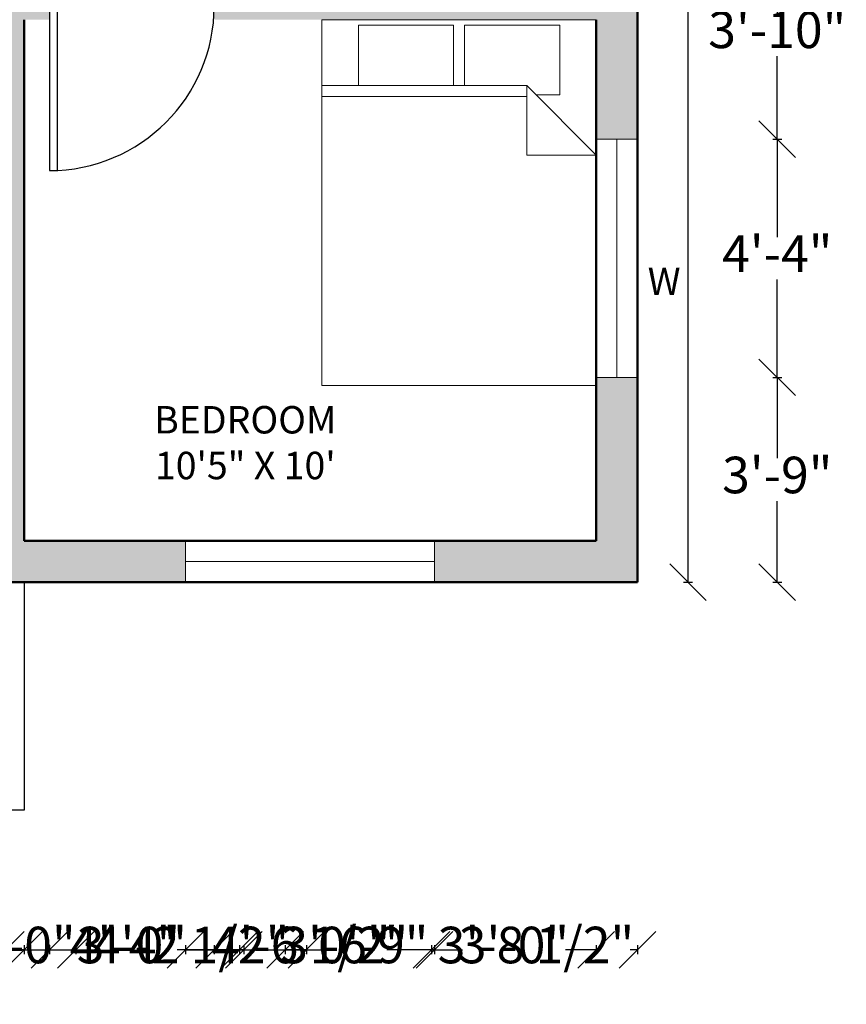
# Model space of a CAD drawing. Units: inches. Extents: x 3121 to 3511, y 1323 to 1998.
# Tile 6 of 10: x 3322 to 3503, y 1323 to 1539. Entities that reach past the tile are written whole.
import ezdxf

# ---------------------------------------------------------------- set-up
doc = ezdxf.new("R2010")
doc.units = ezdxf.units.IN
for name, color, linetype, lineweight in [('A-ANNO-DIMS', 2, 'Continuous', 18), ('A-ANNO-TEXT', 7, 'Continuous', 18), ('A-AREA-IDEN', 7, 'Continuous', 25), ('A-DOOR', 3, 'Continuous', 25), ('A-FLOR', 7, 'Continuous', 25), ('A-FURN', 8, 'Continuous', 18), ('A-GLAZ', 4, 'Continuous', 18), ('A-WALL', 7, 'Continuous', 50), ('A-WALL-PATT', 3, 'Continuous', 13)]:
    doc.layers.add(name, color=color, linetype=linetype, lineweight=lineweight)
doc.styles.get("Standard").update_dxf_attribs({"font": 'arial.ttf'})
doc.dimstyles.new('ISO-25', dxfattribs={"dimtxt": 8, "dimasz": 8, "dimexe": 1, "dimexo": 1, "dimtad": 0, "dimtih": 1, "dimtoh": 1, "dimlunit": 3, "dimtxsty": 'Standard', "dimblk": 'OBLIQUE', "dimcen": 2.5, "dimclrt": 1, "dimadec": 0, "dimazin": 0, "dimtfac": 1, "dimtmove": 0, "dimatfit": 3, "dimfxl": 1, "dimfxlon": 1, "dimarcsym": 0})

# ---------------------------------------------------------------- blocks, each defined once
blk = doc.blocks.new('Bed - Queen')
for p, q in [((0, -80.00003), (0, 0)), ((0, 0), (59.99999, 0)), ((59.99999, 0), (59.99999, -80.00003)), ((7.99999, -1.2), (28.79998, -1.2)), ((7.99999, -14.4), (7.99999, -1.2)), ((28.79998, -1.2), (28.79998, -14.4)), ((31.19999, -1.2), (51.99999, -1.2)), ((31.19999, -14.4), (31.19999, -1.2)), ((51.99999, -1.2), (51.99999, -16.4)), ((0, -14.4), (44.8, -14.4)), ((59.99999, -29.6), (44.8, -14.4)), ((44.8, -14.4), (44.8, -29.6)), ((44.8, -16.8), (0, -16.8)), ((51.99999, -16.4), (46.79936, -16.4)), ((44.8, -29.6), (59.99999, -29.6)), ((59.99999, -80.00003), (0, -80.00003))]:
    blk.add_line(p, q)
blk = doc.blocks.new('*U10')
for p, q in [((0, 0), (0, 6)), ((36, 0), (36, 6))]:
    blk.add_line(p, q)
blk.add_lwpolyline([(0, 0), (0, -36), (1.75, -36), (1.75, 0)], close=True)
blk.add_arc((0, 0), 36, 270, 0)
blk = doc.blocks.new('_Oblique')
at = {"color": 0, "linetype": 'ByBlock', "lineweight": -2}
blk.add_line((-0.5, -0.5), (0.5, 0.5), dxfattribs=at)
blk = doc.blocks.new('*D18')
at = {"layer": 'A-ANNO-DIMS', "color": 0, "lineweight": -2, "transparency": 16777216}
for p, q in [((3466.96, 1955.78), (3468.96, 1955.78)), ((3467.96, 1955.78), (3467.96, 1690.48)), ((3467.96, 1415.78), (3467.96, 1681.09)), ((3466.96, 1415.78), (3468.96, 1415.78))]:
    blk.add_line(p, q, dxfattribs=at)
at = {"layer": 'Defpoints', "color": 0, "transparency": 16777216}
for p in [(3456.92, 1955.78), (3456.92, 1415.78), (3467.96, 1415.78)]:
    blk.add_point(p, dxfattribs=at)
at = {"layer": 'A-ANNO-DIMS', "color": 0, "lineweight": -2, "transparency": 16777216, "xscale": 8, "yscale": 8, "zscale": 8}
for p, rotation in [((3467.96, 1955.78), 90), ((3467.96, 1415.78), 270)]:
    blk.add_blockref('_Oblique', p, dxfattribs=dict(at, rotation=rotation))
at = {"layer": 'A-ANNO-DIMS', "color": 0, "transparency": 16777216, "insert": (3467.96, 1685.78), "char_height": 8, "attachment_point": 5}
blk.add_mtext("45'", dxfattribs=at)
blk = doc.blocks.new('*D34')
at = {"layer": 'A-ANNO-DIMS', "color": 0, "lineweight": -2, "transparency": 16777216}
for p, q in [((3189.92, 1336.37), (3189.92, 1334.37)), ((3189.92, 1335.37), (3242.43, 1335.37)), ((3322.92, 1335.37), (3270.41, 1335.37)), ((3322.92, 1336.37), (3322.92, 1334.37))]:
    blk.add_line(p, q, dxfattribs=at)
at = {"layer": 'Defpoints', "color": 0, "transparency": 16777216}
for p in [(3189.92, 1365.92), (3322.92, 1365.92), (3322.92, 1335.37)]:
    blk.add_point(p, dxfattribs=at)
at = {"layer": 'A-ANNO-DIMS', "color": 0, "lineweight": -2, "transparency": 16777216, "xscale": 8, "yscale": 8, "zscale": 8, "rotation": 180}
blk.add_blockref('_Oblique', (3189.92, 1335.37), dxfattribs=at)
at = {"layer": 'A-ANNO-DIMS', "color": 0, "lineweight": -2, "transparency": 16777216, "xscale": 8, "yscale": 8, "zscale": 8}
blk.add_blockref('_Oblique', (3322.92, 1335.37), dxfattribs=at)
at = {"layer": 'A-ANNO-DIMS', "color": 1, "transparency": 16777216, "insert": (3256.42, 1335.37), "char_height": 8, "attachment_point": 5}
blk.add_mtext('11\'-1"', dxfattribs=at)
blk = doc.blocks.new('*D44')
at = {"layer": 'A-ANNO-DIMS', "color": 0, "lineweight": -2, "transparency": 16777216}
for p, q in [((3486.47, 1460.56), (3488.47, 1460.56)), ((3487.47, 1460.56), (3487.47, 1442.88)), ((3487.47, 1415.78), (3487.47, 1433.46)), ((3486.47, 1415.78), (3488.47, 1415.78))]:
    blk.add_line(p, q, dxfattribs=at)
at = {"layer": 'Defpoints', "color": 0, "transparency": 16777216}
for p in [(3456.92, 1460.56), (3487.47, 1460.56), (3456.92, 1415.78)]:
    blk.add_point(p, dxfattribs=at)
at = {"layer": 'A-ANNO-DIMS', "color": 0, "lineweight": -2, "transparency": 16777216, "xscale": 8, "yscale": 8, "zscale": 8}
for p, rotation in [((3487.47, 1460.56), 90), ((3487.47, 1415.78), 270)]:
    blk.add_blockref('_Oblique', p, dxfattribs=dict(at, rotation=rotation))
at = {"layer": 'A-ANNO-DIMS', "color": 1, "transparency": 16777216, "insert": (3487.47, 1438.17), "char_height": 8, "attachment_point": 5}
blk.add_mtext('3\'-9"', dxfattribs=at)
blk = doc.blocks.new('*D45')
at = {"layer": 'A-ANNO-DIMS', "color": 0, "lineweight": -2, "transparency": 16777216}
for p, q in [((3486.47, 1512.63), (3488.47, 1512.63)), ((3487.47, 1512.63), (3487.47, 1491.22)), ((3487.47, 1460.56), (3487.47, 1481.97)), ((3486.47, 1460.56), (3488.47, 1460.56))]:
    blk.add_line(p, q, dxfattribs=at)
at = {"layer": 'Defpoints', "color": 0, "transparency": 16777216}
for p in [(3456.92, 1512.63), (3487.47, 1512.63), (3456.92, 1460.56)]:
    blk.add_point(p, dxfattribs=at)
at = {"layer": 'A-ANNO-DIMS', "color": 0, "lineweight": -2, "transparency": 16777216, "xscale": 8, "yscale": 8, "zscale": 8}
for p, rotation in [((3487.47, 1512.63), 90), ((3487.47, 1460.56), 270)]:
    blk.add_blockref('_Oblique', p, dxfattribs=dict(at, rotation=rotation))
at = {"layer": 'A-ANNO-DIMS', "color": 1, "transparency": 16777216, "insert": (3487.47, 1486.59), "char_height": 8, "attachment_point": 5}
blk.add_mtext('4\'-4"', dxfattribs=at)
blk = doc.blocks.new('*D46')
at = {"layer": 'A-ANNO-DIMS', "color": 0, "lineweight": -2, "transparency": 16777216}
for p, q in [((3486.47, 1558.43), (3488.47, 1558.43)), ((3487.47, 1558.43), (3487.47, 1540.24)), ((3487.47, 1512.63), (3487.47, 1530.82)), ((3486.47, 1512.63), (3488.47, 1512.63))]:
    blk.add_line(p, q, dxfattribs=at)
at = {"layer": 'Defpoints', "color": 0, "transparency": 16777216}
for p in [(3456.92, 1558.43), (3487.47, 1558.43), (3456.92, 1512.63)]:
    blk.add_point(p, dxfattribs=at)
at = {"layer": 'A-ANNO-DIMS', "color": 0, "lineweight": -2, "transparency": 16777216, "xscale": 8, "yscale": 8, "zscale": 8}
for p, rotation in [((3487.47, 1558.43), 90), ((3487.47, 1512.63), 270)]:
    blk.add_blockref('_Oblique', p, dxfattribs=dict(at, rotation=rotation))
at = {"layer": 'A-ANNO-DIMS', "color": 1, "transparency": 16777216, "insert": (3487.47, 1535.53), "char_height": 8, "attachment_point": 5}
blk.add_mtext('3\'-10"', dxfattribs=at)
blk = doc.blocks.new('*D54')
at = {"layer": 'A-ANNO-DIMS', "color": 0, "lineweight": -2, "transparency": 16777216}
for p, q in [((3310.02, 1336.37), (3310.02, 1334.37)), ((3310.02, 1335.37), (3310.76, 1335.37)), ((3334.16, 1335.37), (3333.42, 1335.37)), ((3334.16, 1336.37), (3334.16, 1334.37))]:
    blk.add_line(p, q, dxfattribs=at)
at = {"layer": 'Defpoints', "color": 0, "transparency": 16777216}
for p in [(3310.02, 1946.78), (3334.16, 1946.78), (3334.16, 1335.37)]:
    blk.add_point(p, dxfattribs=at)
at = {"layer": 'A-ANNO-DIMS', "color": 0, "lineweight": -2, "transparency": 16777216, "xscale": 8, "yscale": 8, "zscale": 8, "rotation": 180}
blk.add_blockref('_Oblique', (3310.02, 1335.37), dxfattribs=at)
at = {"layer": 'A-ANNO-DIMS', "color": 0, "lineweight": -2, "transparency": 16777216, "xscale": 8, "yscale": 8, "zscale": 8}
blk.add_blockref('_Oblique', (3334.16, 1335.37), dxfattribs=at)
at = {"layer": 'A-ANNO-DIMS', "color": 1, "transparency": 16777216, "insert": (3322.09, 1335.37), "char_height": 8, "attachment_point": 5}
blk.add_mtext('2\'-0"', dxfattribs=at)
blk = doc.blocks.new('*D55')
at = {"layer": 'A-ANNO-DIMS', "color": 0, "lineweight": -2, "transparency": 16777216}
for p, q in [((3334.16, 1336.37), (3334.16, 1334.37)), ((3334.16, 1335.37), (3338.62, 1335.37)), ((3384.56, 1335.37), (3380.1, 1335.37)), ((3384.56, 1336.37), (3384.56, 1334.37))]:
    blk.add_line(p, q, dxfattribs=at)
at = {"layer": 'Defpoints', "color": 0, "transparency": 16777216}
for p in [(3334.16, 1946.78), (3384.56, 1946.78), (3384.56, 1335.37)]:
    blk.add_point(p, dxfattribs=at)
at = {"layer": 'A-ANNO-DIMS', "color": 0, "lineweight": -2, "transparency": 16777216, "xscale": 8, "yscale": 8, "zscale": 8, "rotation": 180}
blk.add_blockref('_Oblique', (3334.16, 1335.37), dxfattribs=at)
at = {"layer": 'A-ANNO-DIMS', "color": 0, "lineweight": -2, "transparency": 16777216, "xscale": 8, "yscale": 8, "zscale": 8}
blk.add_blockref('_Oblique', (3384.56, 1335.37), dxfattribs=at)
at = {"layer": 'A-ANNO-DIMS', "color": 1, "transparency": 16777216, "insert": (3359.36, 1335.37), "char_height": 8, "attachment_point": 5}
blk.add_mtext('4\'-2 1/2"', dxfattribs=at)
blk = doc.blocks.new('*D56')
at = {"layer": 'A-ANNO-DIMS', "color": 0, "lineweight": -2, "transparency": 16777216}
for p, q in [((3358.15, 1336.37), (3358.15, 1334.37)), ((3358.15, 1335.37), (3364.61, 1335.37)), ((3412.54, 1335.37), (3406.09, 1335.37)), ((3412.54, 1336.37), (3412.54, 1334.37))]:
    blk.add_line(p, q, dxfattribs=at)
at = {"layer": 'Defpoints', "color": 0, "transparency": 16777216}
for p in [(3358.15, 1415.78), (3412.54, 1415.78), (3412.54, 1335.37)]:
    blk.add_point(p, dxfattribs=at)
at = {"layer": 'A-ANNO-DIMS', "color": 0, "lineweight": -2, "transparency": 16777216, "xscale": 8, "yscale": 8, "zscale": 8, "rotation": 180}
blk.add_blockref('_Oblique', (3358.15, 1335.37), dxfattribs=at)
at = {"layer": 'A-ANNO-DIMS', "color": 0, "lineweight": -2, "transparency": 16777216, "xscale": 8, "yscale": 8, "zscale": 8}
blk.add_blockref('_Oblique', (3412.54, 1335.37), dxfattribs=at)
at = {"layer": 'A-ANNO-DIMS', "color": 1, "transparency": 16777216, "insert": (3385.35, 1335.37), "char_height": 8, "attachment_point": 5}
blk.add_mtext('4\'-6 1/2"', dxfattribs=at)
blk = doc.blocks.new('*D57')
at = {"layer": 'A-ANNO-DIMS', "color": 0, "lineweight": -2, "transparency": 16777216}
for p, q in [((3412.54, 1336.37), (3412.54, 1334.37)), ((3412.54, 1335.37), (3414.15, 1335.37)), ((3456.92, 1335.37), (3455.31, 1335.37)), ((3456.92, 1336.37), (3456.92, 1334.37))]:
    blk.add_line(p, q, dxfattribs=at)
at = {"layer": 'Defpoints', "color": 0, "transparency": 16777216}
for p in [(3412.54, 1415.78), (3456.92, 1415.78), (3456.92, 1335.37)]:
    blk.add_point(p, dxfattribs=at)
at = {"layer": 'A-ANNO-DIMS', "color": 0, "lineweight": -2, "transparency": 16777216, "xscale": 8, "yscale": 8, "zscale": 8, "rotation": 180}
blk.add_blockref('_Oblique', (3412.54, 1335.37), dxfattribs=at)
at = {"layer": 'A-ANNO-DIMS', "color": 0, "lineweight": -2, "transparency": 16777216, "xscale": 8, "yscale": 8, "zscale": 8}
blk.add_blockref('_Oblique', (3456.92, 1335.37), dxfattribs=at)
at = {"layer": 'A-ANNO-DIMS', "color": 1, "transparency": 16777216, "insert": (3434.73, 1335.37), "char_height": 8, "attachment_point": 5}
blk.add_mtext('3\'-8 1/2"', dxfattribs=at)
blk = doc.blocks.new('*D59')
at = {"layer": 'A-ANNO-DIMS', "color": 0, "lineweight": -2, "transparency": 16777216}
for p, q in [((3318.92, 1336.37), (3318.92, 1334.37)), ((3318.92, 1335.37), (3333.5, 1335.37)), ((3370.92, 1335.37), (3356.34, 1335.37)), ((3370.92, 1336.37), (3370.92, 1334.37))]:
    blk.add_line(p, q, dxfattribs=at)
at = {"layer": 'Defpoints', "color": 0, "transparency": 16777216}
for p in [(3318.92, 1752.23), (3370.92, 1748.78), (3370.92, 1335.37)]:
    blk.add_point(p, dxfattribs=at)
at = {"layer": 'A-ANNO-DIMS', "color": 0, "lineweight": -2, "transparency": 16777216, "xscale": 8, "yscale": 8, "zscale": 8, "rotation": 180}
blk.add_blockref('_Oblique', (3318.92, 1335.37), dxfattribs=at)
at = {"layer": 'A-ANNO-DIMS', "color": 0, "lineweight": -2, "transparency": 16777216, "xscale": 8, "yscale": 8, "zscale": 8}
blk.add_blockref('_Oblique', (3370.92, 1335.37), dxfattribs=at)
at = {"layer": 'A-ANNO-DIMS', "color": 1, "transparency": 16777216, "insert": (3344.92, 1335.37), "char_height": 8, "attachment_point": 5}
blk.add_mtext('4\'-4"', dxfattribs=at)
blk = doc.blocks.new('*D63')
at = {"layer": 'A-ANNO-DIMS', "color": 0, "lineweight": -2, "transparency": 16777216}
for p, q in [((3370.92, 1336.37), (3370.92, 1334.37)), ((3370.92, 1335.37), (3379.92, 1335.37)), ((3379.92, 1336.37), (3379.92, 1334.37)), ((3379.92, 1335.37), (3387.92, 1335.37))]:
    blk.add_line(p, q, dxfattribs=at)
at = {"layer": 'Defpoints', "color": 0, "transparency": 16777216}
for p in [(3370.92, 1748.78), (3379.92, 1748.78), (3379.92, 1335.37)]:
    blk.add_point(p, dxfattribs=at)
at = {"layer": 'A-ANNO-DIMS', "color": 0, "lineweight": -2, "transparency": 16777216, "xscale": 8, "yscale": 8, "zscale": 8, "rotation": 180}
blk.add_blockref('_Oblique', (3370.92, 1335.37), dxfattribs=at)
at = {"layer": 'A-ANNO-DIMS', "color": 0, "lineweight": -2, "transparency": 16777216, "xscale": 8, "yscale": 8, "zscale": 8}
blk.add_blockref('_Oblique', (3379.92, 1335.37), dxfattribs=at)
at = {"layer": 'A-ANNO-DIMS', "color": 1, "transparency": 16777216, "insert": (3399.18, 1335.37), "char_height": 8, "attachment_point": 5}
blk.add_mtext('0\'-9"', dxfattribs=at)
blk = doc.blocks.new('*D64')
at = {"layer": 'A-ANNO-DIMS', "color": 0, "lineweight": -2, "transparency": 16777216}
for p, q in [((3411.92, 1336.37), (3411.92, 1334.37)), ((3411.92, 1335.37), (3418.66, 1335.37)), ((3447.92, 1335.37), (3441.17, 1335.37)), ((3447.92, 1336.37), (3447.92, 1334.37))]:
    blk.add_line(p, q, dxfattribs=at)
at = {"layer": 'Defpoints', "color": 0, "transparency": 16777216}
for p in [(3411.92, 1638.28), (3447.92, 1638.28), (3447.92, 1335.37)]:
    blk.add_point(p, dxfattribs=at)
at = {"layer": 'A-ANNO-DIMS', "color": 0, "lineweight": -2, "transparency": 16777216, "xscale": 8, "yscale": 8, "zscale": 8, "rotation": 180}
blk.add_blockref('_Oblique', (3411.92, 1335.37), dxfattribs=at)
at = {"layer": 'A-ANNO-DIMS', "color": 0, "lineweight": -2, "transparency": 16777216, "xscale": 8, "yscale": 8, "zscale": 8}
blk.add_blockref('_Oblique', (3447.92, 1335.37), dxfattribs=at)
at = {"layer": 'A-ANNO-DIMS', "color": 1, "transparency": 16777216, "insert": (3429.92, 1335.37), "char_height": 8, "attachment_point": 5}
blk.add_mtext('3\'-0"', dxfattribs=at)
blk = doc.blocks.new('*D72')
at = {"layer": 'A-ANNO-DIMS', "color": 0, "lineweight": -2, "transparency": 16777216}
for p, q in [((3328.42, 1336.37), (3328.42, 1334.37)), ((3328.42, 1335.37), (3335.16, 1335.37)), ((3364.42, 1335.37), (3357.67, 1335.37)), ((3364.42, 1336.37), (3364.42, 1334.37))]:
    blk.add_line(p, q, dxfattribs=at)
at = {"layer": 'Defpoints', "color": 0, "transparency": 16777216}
for p in [(3328.42, 1538.78), (3364.42, 1538.78), (3364.42, 1335.37)]:
    blk.add_point(p, dxfattribs=at)
at = {"layer": 'A-ANNO-DIMS', "color": 0, "lineweight": -2, "transparency": 16777216, "xscale": 8, "yscale": 8, "zscale": 8, "rotation": 180}
blk.add_blockref('_Oblique', (3328.42, 1335.37), dxfattribs=at)
at = {"layer": 'A-ANNO-DIMS', "color": 0, "lineweight": -2, "transparency": 16777216, "xscale": 8, "yscale": 8, "zscale": 8}
blk.add_blockref('_Oblique', (3364.42, 1335.37), dxfattribs=at)
at = {"layer": 'A-ANNO-DIMS', "color": 1, "transparency": 16777216, "insert": (3346.42, 1335.37), "char_height": 8, "attachment_point": 5}
blk.add_mtext('3\'-0"', dxfattribs=at)
blk = doc.blocks.new('*D75')
at = {"layer": 'A-ANNO-DIMS', "color": 0, "lineweight": -2, "transparency": 16777216}
for p, q in [((3369.92, 1336.37), (3369.92, 1334.37)), ((3369.92, 1335.37), (3379.66, 1335.37)), ((3411.92, 1335.37), (3402.17, 1335.37)), ((3411.92, 1336.37), (3411.92, 1334.37))]:
    blk.add_line(p, q, dxfattribs=at)
at = {"layer": 'Defpoints', "color": 0, "transparency": 16777216}
for p in [(3369.92, 1703.78), (3411.92, 1703.78), (3411.92, 1335.37)]:
    blk.add_point(p, dxfattribs=at)
at = {"layer": 'A-ANNO-DIMS', "color": 0, "lineweight": -2, "transparency": 16777216, "xscale": 8, "yscale": 8, "zscale": 8, "rotation": 180}
blk.add_blockref('_Oblique', (3369.92, 1335.37), dxfattribs=at)
at = {"layer": 'A-ANNO-DIMS', "color": 0, "lineweight": -2, "transparency": 16777216, "xscale": 8, "yscale": 8, "zscale": 8}
blk.add_blockref('_Oblique', (3411.92, 1335.37), dxfattribs=at)
at = {"layer": 'A-ANNO-DIMS', "color": 1, "transparency": 16777216, "insert": (3390.92, 1335.37), "char_height": 8, "attachment_point": 5}
blk.add_mtext('3\'-6"', dxfattribs=at)

msp = doc.modelspace()

# ---------------------------------------------------------------- hatches: boundary and pattern name
at = {"layer": 'A-WALL-PATT'}
h = msp.add_hatch(color=256, dxfattribs=at)
h.dxf.hatch_style = 1
h.paths.add_polyline_path([(3274.023, 1955.784), (3189.918, 1955.784), (3189.918, 1910.219), (3198.918, 1910.219), (3198.918, 1946.784), (3259.023, 1946.784), (3259.023, 1921.61), (3261.023, 1921.61), (3261.023, 1946.784), (3274.023, 1946.784)])
h.paths.add_polyline_path([(3327.918, 1946.784), (3334.156, 1946.784), (3334.156, 1955.784), (3310.023, 1955.784), (3310.023, 1946.784), (3318.918, 1946.784), (3318.918, 1929.796), (3311.644, 1929.796), (3311.644, 1927.007), (3324.033, 1927.007), (3324.033, 1871.381), (3311.644, 1871.381), (3311.644, 1868.381), (3318.918, 1868.381), (3318.918, 1853.784), (3327.918, 1853.784)])
h.paths.add_polyline_path([(3456.918, 1955.784), (3384.562, 1955.784), (3384.562, 1946.784), (3447.918, 1946.784), (3447.918, 1877.779), (3456.918, 1877.779)])
h.paths.add_polyline_path([(3456.918, 1835.782), (3447.918, 1835.782), (3447.918, 1814.784), (3414.918, 1814.784), (3414.918, 1803.784), (3447.918, 1803.784), (3447.918, 1793.443), (3456.918, 1793.443)])
h.paths.add_polyline_path([(3456.918, 1558.434), (3447.918, 1558.434), (3447.918, 1547.784), (3375.918, 1547.784), (3375.918, 1598.784), (3378.918, 1598.784), (3378.918, 1602.284), (3375.918, 1602.284), (3375.918, 1674.284), (3369.918, 1674.284), (3369.918, 1547.784), (3364.418, 1547.784), (3364.418, 1538.784), (3447.918, 1538.784), (3447.918, 1512.628), (3456.918, 1512.628)])
h.paths.add_polyline_path([(3456.918, 1460.558), (3447.918, 1460.558), (3447.918, 1424.784), (3412.543, 1424.784), (3412.543, 1415.784), (3456.918, 1415.784)])
h.paths.add_polyline_path([(3358.149, 1424.784), (3322.918, 1424.784), (3322.918, 1538.784), (3328.418, 1538.784), (3328.418, 1547.784), (3308.208, 1547.784), (3308.208, 1538.784), (3318.918, 1538.784), (3318.918, 1424.784), (3311.328, 1424.784), (3311.328, 1415.784), (3358.149, 1415.784)])
h.paths.add_polyline_path([(3207.562, 1547.784), (3198.918, 1547.784), (3198.918, 1607.327), (3189.918, 1607.327), (3189.918, 1513.073), (3198.918, 1513.073), (3198.918, 1538.784), (3207.562, 1538.784)])
h.paths.add_polyline_path([(3198.918, 1461.548), (3189.918, 1461.548), (3189.918, 1415.784), (3209.892, 1415.784), (3209.892, 1424.784), (3198.918, 1424.784)])
h.paths.add_polyline_path([(3272.208, 1547.784), (3238.766, 1547.784), (3238.766, 1538.784), (3272.208, 1538.784)])
h.paths.add_polyline_path([(3261.023, 1748.784), (3198.918, 1748.784), (3198.918, 1768.387), (3189.918, 1768.387), (3189.918, 1692.279), (3198.918, 1692.279), (3198.918, 1739.784), (3261.023, 1739.784)])
h.paths.add_polyline_path([(3198.918, 1856.171), (3189.918, 1856.171), (3189.918, 1808.331), (3198.918, 1808.331), (3198.918, 1821.074), (3261.023, 1821.074), (3261.023, 1862.309), (3259.023, 1862.309), (3259.023, 1825.074), (3198.918, 1825.074)])

# ---------------------------------------------------------------- linework, layer by layer
at = {"layer": 'A-FLOR'}
msp.add_lwpolyline([(3322.918, 1415.784), (3322.918, 1365.917), (3189.918, 1365.917), (3189.918, 1415.784)], dxfattribs=at)
at = {"layer": 'A-GLAZ'}
for p, q in [((3447.918, 1512.628), (3456.918, 1512.628)), ((3452.418, 1512.628), (3452.418, 1460.558)), ((3447.918, 1460.558), (3456.918, 1460.558)), ((3358.149, 1424.784), (3358.149, 1415.784)), ((3412.543, 1424.784), (3412.543, 1415.784)), ((3358.149, 1420.284), (3412.543, 1420.284))]:
    msp.add_line(p, q, dxfattribs=at)
at = {"layer": 'A-WALL'}
for p, q in [((3456.918, 1415.784), (3456.918, 1955.784)), ((3322.918, 1424.784), (3322.918, 1538.784)), ((3447.918, 1424.784), (3447.918, 1538.784)), ((3322.918, 1424.784), (3447.918, 1424.784)), ((3311.328, 1415.784), (3456.918, 1415.784))]:
    msp.add_line(p, q, dxfattribs=at)

# ---------------------------------------------------------------- block references
at = {"layer": 'A-DOOR'}
msp.add_blockref('*U10', (3328.418, 1541.784), dxfattribs=at)
at = {"layer": 'A-FURN'}
msp.add_blockref('Bed - Queen', (3387.918, 1538.784), dxfattribs=at)

# ---------------------------------------------------------------- texts
at = {"layer": 'A-ANNO-TEXT', "insert": (3456.532, 1484.573), "char_height": 6, "attachment_point": 1}
msp.add_mtext_dynamic_manual_height_columns('\\pxqc;W', width=12.42925, gutter_width=12.5, heights=[0], dxfattribs=at)
at = {"layer": 'A-AREA-IDEN', "insert": (3336.401, 1454.28), "char_height": 6, "attachment_point": 1}
msp.add_mtext_dynamic_manual_height_columns('\\pxqc;BEDROOM\\P10\'5" X 10\'', width=69.63762, gutter_width=12.5, heights=[0], dxfattribs=at)

# ---------------------------------------------------------------- dimensions: what is measured, and where the dimension line sits
at = {"layer": 'A-ANNO-DIMS'}
for base, p1, p2, override, picture, middle in [((3467.957, 1415.784), (3456.918, 1955.784), (3456.918, 1415.784), {"dimclrd": 0, "dimclre": 0, "dimclrt": 0}, '*D18', (3467.957, 1685.784)), ((3487.468, 1558.434), (3456.918, 1512.628), (3456.918, 1558.434), {"dimdec": 1, "dimlfac": 1, "dimrnd": 0, "dimzin": 1, "dimdsep": 46, "dimlunit": 4, "dimfrac": 2}, '*D46', (3487.468, 1535.531)), ((3487.468, 1512.628), (3456.918, 1460.558), (3456.918, 1512.628), {"dimdec": 1, "dimlfac": 1, "dimrnd": 0, "dimzin": 1, "dimdsep": 46, "dimlunit": 4, "dimfrac": 2}, '*D45', (3487.468, 1486.593)), ((3487.468, 1460.558), (3456.918, 1415.784), (3456.918, 1460.558), {"dimdec": 1, "dimlfac": 1, "dimrnd": 0, "dimzin": 1, "dimdsep": 46, "dimlunit": 4, "dimfrac": 2}, '*D44', (3487.468, 1438.171))]:
    dim = msp.add_linear_dim(base=base, p1=p1, p2=p2, angle=90, dimstyle='ISO-25', override=override, dxfattribs=at)
    dim.commit()
    dim.dimension.update_dxf_attribs({"geometry": picture, "text_midpoint": middle})
for base, p1, p2, picture, middle in [((3334.156, 1335.367), (3310.023, 1946.784), (3334.156, 1946.784), '*D54', (3322.089, 1335.367)), ((3384.562, 1335.367), (3334.156, 1946.784), (3384.562, 1946.784), '*D55', (3359.359, 1335.367)), ((3370.918, 1335.367), (3318.918, 1752.226), (3370.918, 1748.784), '*D59', (3344.918, 1335.367)), ((3379.918, 1335.367), (3370.918, 1748.784), (3379.918, 1748.784), '*D63', (3399.176, 1335.367)), ((3411.918, 1335.367), (3369.918, 1703.784), (3411.918, 1703.784), '*D75', (3390.918, 1335.367)), ((3447.918, 1335.367), (3411.918, 1638.284), (3447.918, 1638.284), '*D64', (3429.918, 1335.367)), ((3364.418, 1335.367), (3328.418, 1538.784), (3364.418, 1538.784), '*D72', (3346.418, 1335.367)), ((3412.543, 1335.367), (3358.149, 1415.784), (3412.543, 1415.784), '*D56', (3385.346, 1335.367)), ((3456.918, 1335.367), (3412.543, 1415.784), (3456.918, 1415.784), '*D57', (3434.731, 1335.367)), ((3322.918, 1335.367), (3189.918, 1365.917), (3322.918, 1365.917), '*D34', (3256.418, 1335.367))]:
    dim = msp.add_linear_dim(base=base, p1=p1, p2=p2, dimstyle='ISO-25', override={"dimdec": 1, "dimlfac": 1, "dimrnd": 0, "dimzin": 1, "dimdsep": 46, "dimlunit": 4, "dimfrac": 2}, dxfattribs=at)
    dim.commit()
    dim.dimension.update_dxf_attribs({"geometry": picture, "text_midpoint": middle})

doc.saveas('drawing.dxf')
